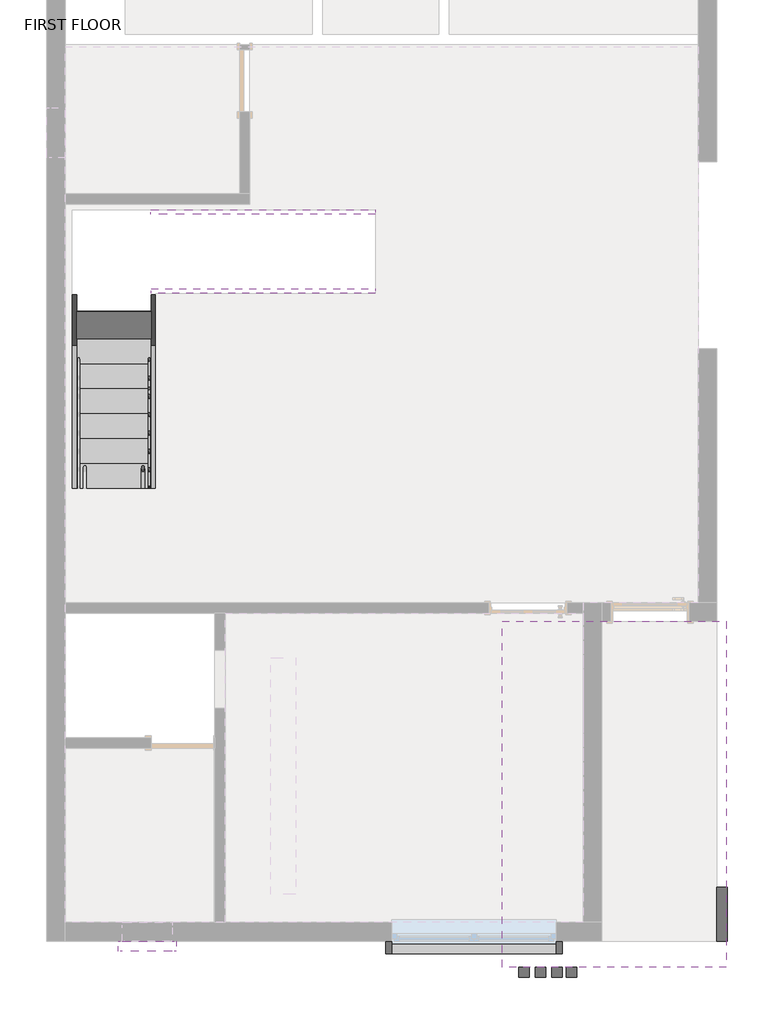
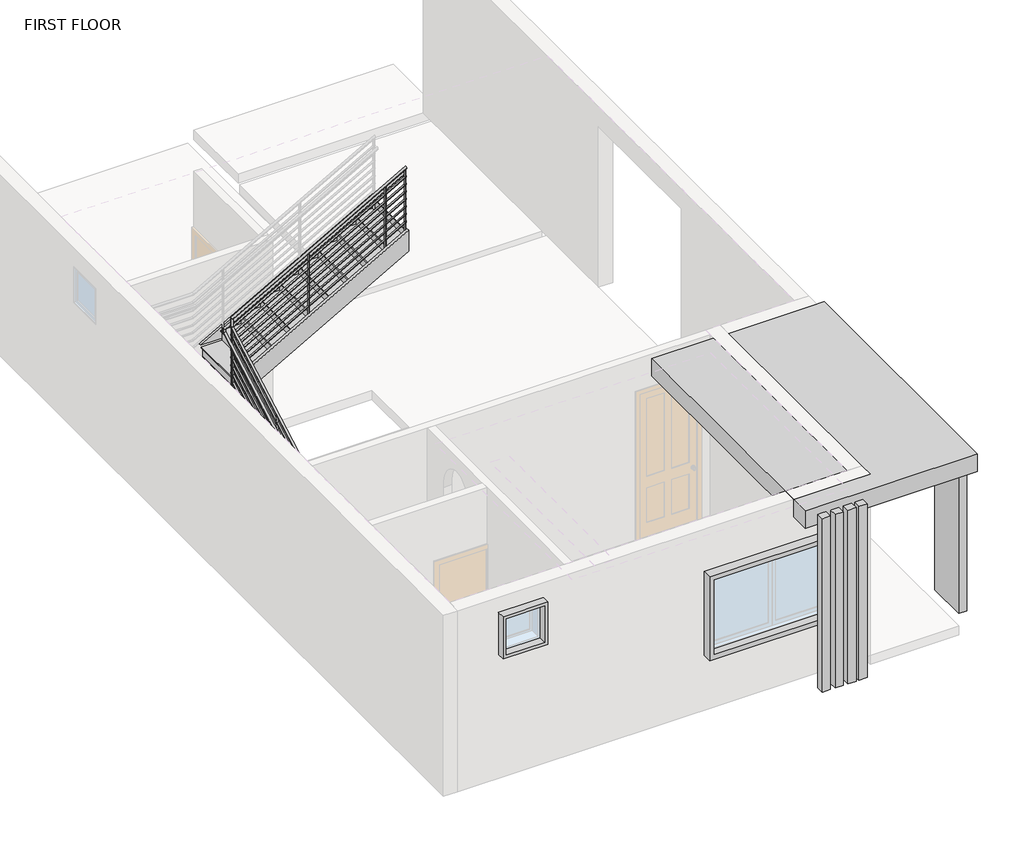
# One storey, part 3 of 3: 5 proxies, 4 members, 1 railing, 1 stair flight.
"""IFC4 building model written with IfcOpenShell, lengths in millimetres."""

from ifc_helpers import new_model, si_unit, frame, origin, place, context, project, spatial, polyline, circle_curve, ellipse_curve, outline, extrude, transform, mapped, element, save
from ifc_brep_helpers import plane_surface, cylinder_surface, advanced_brep
from components import generic_models_1_generic_models_1_e6ddf01a, generic_models_3_generic_models_3_ef4d42f5, generic_models_5_generic_models_5_8773877a, generic_models_7_generic_models_7_fd49988f, generic_models_9_generic_models_9_50e4b17c, stair_flight_ebba5fc4

model = new_model("IFC4")

# Units and contexts
model_context = context("Model", 3, world=origin())
ifc_project = project(units=[si_unit("LENGTHUNIT", "METRE", prefix="MILLI")], contexts=[model_context])

# Site, building, storey
site = spatial("IfcSite", under=ifc_project)
building = spatial("IfcBuilding", under=site)
storey = spatial("IfcBuildingStorey", under=building, Name="FIRST FLOOR", Elevation=3352.8)

# Proxies
placement = place(None, origin())
generic_models_1_generic_models_1_shape = generic_models_1_generic_models_1_e6ddf01a(model_context)
element("IfcBuildingElementProxy", 1, Name="Generic Models 1 : Generic Models 1", ObjectType="Generic Models 1 : Generic Models 1", at=placement, inside=storey, context=model_context, shape_type="MappedRepresentation", body=[
    mapped(generic_models_1_generic_models_1_shape, transform((0.0, 0.0, 0.0), x_axis=(1.0, 0.0, 0.0), y_axis=(0.0, 1.0, 0.0), z_axis=(0.0, 0.0, 1.0))),
])
generic_models_3_generic_models_3_shape = generic_models_3_generic_models_3_ef4d42f5(model_context)
element("IfcBuildingElementProxy", 2, Name="Generic Models 3 : Generic Models 3", ObjectType="Generic Models 3 : Generic Models 3", at=placement, inside=storey, context=model_context, shape_type="MappedRepresentation", body=[
    mapped(generic_models_3_generic_models_3_shape, transform((0.0, 0.0, 0.0), x_axis=(1.0, 0.0, 0.0), y_axis=(0.0, 1.0, 0.0), z_axis=(0.0, 0.0, 1.0))),
])
generic_models_5_generic_models_5_shape = generic_models_5_generic_models_5_8773877a(model_context)
element("IfcBuildingElementProxy", 3, Name="Generic Models 5 : Generic Models 5", ObjectType="Generic Models 5 : Generic Models 5", at=placement, inside=storey, context=model_context, shape_type="MappedRepresentation", body=[
    mapped(generic_models_5_generic_models_5_shape, transform((0.0, 0.0, 0.0), x_axis=(1.0, 0.0, 0.0), y_axis=(0.0, 1.0, 0.0), z_axis=(0.0, 0.0, 1.0))),
])
generic_models_7_generic_models_7_shape = generic_models_7_generic_models_7_fd49988f(model_context)
element("IfcBuildingElementProxy", 4, Name="Generic Models 7 : Generic Models 7", ObjectType="Generic Models 7 : Generic Models 7", at=placement, inside=storey, context=model_context, shape_type="MappedRepresentation", body=[
    mapped(generic_models_7_generic_models_7_shape, transform((0.0, 0.0, 0.0), x_axis=(1.0, 0.0, 0.0), y_axis=(0.0, 1.0, 0.0), z_axis=(0.0, 0.0, 1.0))),
])
generic_models_9_generic_models_9_shape = generic_models_9_generic_models_9_50e4b17c(model_context)
element("IfcBuildingElementProxy", 5, Name="Generic Models 9 : Generic Models 9", ObjectType="Generic Models 9 : Generic Models 9", at=placement, inside=storey, context=model_context, shape_type="MappedRepresentation", body=[
    mapped(generic_models_9_generic_models_9_shape, transform((0.0, 0.0, 0.0), x_axis=(1.0, 0.0, 0.0), y_axis=(0.0, 1.0, 0.0), z_axis=(0.0, 0.0, 1.0))),
])

# Members
element("IfcMember", 6, ObjectType="Stringer - 2\" Width", at=placement, inside=storey, context=model_context, shape_type="SweptSolid", body=[
    extrude(outline(polyline([(1771.427543, 3352.8), (1771.427543, 3561.3575825), (3600.227543, 4597.6775825), (4218.4673554, 4597.6775825), (2021.6245627, 3352.8), (1771.427543, 3352.8)])), frame((-6992.4757327, 0.0, 0.0), z_axis=(1.0, 0.0, 0.0), x_axis=(0.0, 1.0, 0.0)), (0.0, 0.0, 1.0), 50.8),
])
element("IfcMember", 7, ObjectType="Stringer - 2\" Width", at=placement, inside=storey, context=model_context, shape_type="SweptSolid", body=[
    extrude(outline(polyline([(5110.9416888, -5417.6757327), (6319.9816888, -3284.0757327), (6670.3175825, -3284.0757327), (5110.9416888, -6035.915545), (5110.9416888, -5417.6757327)])), frame((0.0, 5124.227543, 0.0), z_axis=(0.0, 1.0, 0.0), x_axis=(0.0, 0.0, 1.0)), (0.0, 0.0, 1.0), 50.8),
])
element("IfcMember", 8, ObjectType="Stringer - 2\" Width", at=placement, inside=storey, context=model_context, shape_type="SweptSolid", body=[
    extrude(outline(polyline([(1771.427543, 3352.8), (1771.427543, 3561.3575825), (4159.027543, 4914.3309158), (4159.027543, 4563.9950222), (2021.6245627, 3352.8), (1771.427543, 3352.8)])), frame((-6027.2757327, 0.0, 0.0), z_axis=(1.0, 0.0, 0.0), x_axis=(0.0, 1.0, 0.0)), (0.0, 0.0, 1.0), 50.8),
])
element("IfcMember", 9, ObjectType="Stringer - 2\" Width", at=placement, inside=storey, context=model_context, shape_type="SweptSolid", body=[
    extrude(outline(polyline([(5115.8375825, -6027.2757327), (4765.5016888, -6027.2757327), (6319.9816888, -3284.0757327), (6670.3175825, -3284.0757327), (5115.8375825, -6027.2757327)])), frame((0.0, 4159.027543, 0.0), z_axis=(0.0, 1.0, 0.0), x_axis=(0.0, 0.0, 1.0)), (0.0, 0.0, 1.0), 50.8),
])

# Railing
element("IfcRailing", 10, ObjectType="Guardrail - Pipe", at=placement, inside=storey, context=model_context, shape_type="AdvancedBrep", body=[
    advanced_brep(
    [(-6109.8257327, 1771.427543, 4418.0240066), (-6147.9257327, 1771.427543, 4418.0240066), (-6109.8257327, 4311.427543, 5857.35734), (-6147.9257327, 4311.427543, 5857.35734)],
    [
        (0, 1, ellipse_curve(frame((-6128.8757327, 1771.427543, 4418.0240066), z_axis=(0.0, -1.0, 0.0), x_axis=(0.0, 0.0, -0.9999999999999999)), 21.8959934, 19.05)),
        (1, 0, ellipse_curve(frame((-6128.8757327, 1771.427543, 4418.0240066), z_axis=(0.0, -1.0, 0.0), x_axis=(0.0, 0.0, -0.9999999999999999)), 21.8959934, 19.05)),
        (2, 3, ellipse_curve(frame((-6128.8757327, 4311.427543, 5857.35734), z_axis=(0.0, 0.5034815925230599, 0.864005952520261), x_axis=(0.0, -0.864005952520261, 0.5034815925230601)), 22.0484592, 19.05)),
        (3, 2, ellipse_curve(frame((-6128.8757327, 4311.427543, 5857.35734), z_axis=(0.0, 0.5034815925230599, 0.864005952520261), x_axis=(0.0, -0.864005952520261, 0.5034815925230601)), 22.0484592, 19.05)),
        (0, 2),
        (3, 1),
    ],
    [
        plane_surface(frame((-6128.8757327, 1771.427543, 4439.92), z_axis=(0.0, -1.0, 0.0), x_axis=(0.0, 0.0, 1.0))),
        plane_surface(frame((-6128.8757327, 4292.377543, 5868.4583333), z_axis=(0.0, 0.5034815925230599, 0.864005952520261), x_axis=(1.0, 0.0, 0.0))),
        cylinder_surface(frame((-6128.8757327, 1780.8194325, 4423.3460774), z_axis=(0.0, -0.8700221858486086, -0.49301257198088694), x_axis=(-1.0, 0.0, 0.0)), 19.05),
    ],
    [
        (0, [[1, 2]]),
        (1, [[3, 4]]),
        (2, [[-1, 5, -4, 6]]),
        (2, [[-2, -6, -3, -5]]),
    ],
),
    advanced_brep(
    [(-6109.8257327, 4313.9036203, 5855.9144571), (-6147.9257327, 4313.9036203, 5855.9144571), (-6109.8257327, 4313.9036203, 5903.82968), (-6147.9257327, 4313.9036203, 5926.0316667)],
    [
        (0, 1, ellipse_curve(frame((-6128.8757327, 4313.9036203, 5855.9144571), z_axis=(0.0, -0.5034815925230599, -0.864005952520261), x_axis=(0.0, 0.8640059525202612, -0.5034815925230599)), 22.0484592, 19.05)),
        (1, 0, ellipse_curve(frame((-6128.8757327, 4313.9036203, 5855.9144571), z_axis=(0.0, -0.5034815925230599, -0.864005952520261), x_axis=(0.0, 0.8640059525202612, -0.5034815925230599)), 22.0484592, 19.05)),
        (2, 3, ellipse_curve(frame((-6128.8757327, 4313.9036203, 5914.9306733), z_axis=(0.5034815925230599, 0.0, 0.864005952520261), x_axis=(0.8640059525202612, 0.0, -0.5034815925230599)), 22.0484592, 19.05)),
        (3, 2, ellipse_curve(frame((-6128.8757327, 4313.9036203, 5914.9306733), z_axis=(0.5034815925230599, 0.0, 0.864005952520261), x_axis=(0.8640059525202612, 0.0, -0.5034815925230599)), 22.0484592, 19.05)),
        (0, 2),
        (3, 1),
    ],
    [
        plane_surface(frame((-6128.8757327, 4311.427543, 5857.35734), z_axis=(0.0, -0.5034815925230599, -0.864005952520261), x_axis=(1.0, 0.0, 0.0))),
        plane_surface(frame((-6128.8757327, 4311.427543, 5914.9306733), z_axis=(0.5034815925230599, 0.0, 0.864005952520261), x_axis=(0.864005952520261, 0.0, -0.5034815925230599))),
        cylinder_surface(frame((-6128.8757327, 4313.9036203, 5857.35734), z_axis=(0.0, 0.0, -1.0), x_axis=(-1.0, 0.0, 0.0)), 19.05),
    ],
    [
        (0, [[1, 2]]),
        (1, [[3, 4]]),
        (2, [[-1, 5, -4, 6]]),
        (2, [[-2, -6, -3, -5]]),
    ],
),
    advanced_brep(
    [(-6128.8757327, 4292.377543, 5914.9306733), (-6128.8757327, 4330.477543, 5914.9306733), (-3284.0757327, 4292.377543, 7526.9840066), (-3284.0757327, 4330.477543, 7526.9840066)],
    [
        (0, 1, ellipse_curve(frame((-6128.8757327, 4311.427543, 5914.9306733), z_axis=(-0.5034815925230599, 0.0, -0.864005952520261), x_axis=(-0.864005952520261, 0.0, 0.5034815925230601)), 22.0484592, 19.05)),
        (1, 0, ellipse_curve(frame((-6128.8757327, 4311.427543, 5914.9306733), z_axis=(-0.5034815925230599, 0.0, -0.864005952520261), x_axis=(-0.864005952520261, 0.0, 0.5034815925230601)), 22.0484592, 19.05)),
        (2, 3, ellipse_curve(frame((-3284.0757327, 4311.427543, 7526.9840066), z_axis=(1.0, 0.0, 0.0), x_axis=(0.0, 0.0, -0.9999999999999999)), 21.8959934, 19.05)),
        (3, 2, ellipse_curve(frame((-3284.0757327, 4311.427543, 7526.9840066), z_axis=(1.0, 0.0, 0.0), x_axis=(0.0, 0.0, -0.9999999999999999)), 21.8959934, 19.05)),
        (0, 2),
        (3, 1),
    ],
    [
        plane_surface(frame((-6147.9257327, 4311.427543, 5926.0316667), z_axis=(-0.5034815925230599, 0.0, -0.864005952520261), x_axis=(0.864005952520261, 0.0, -0.5034815925230599))),
        plane_surface(frame((-3284.0757327, 4311.427543, 7548.88), z_axis=(1.0, 0.0, 0.0), x_axis=(0.0, 1.0, 0.0))),
        cylinder_surface(frame((-6138.5338432, 4311.427543, 5909.457744), z_axis=(-0.8700221858486086, 0.0, -0.49301257198088694), x_axis=(0.0, 1.0, 0.0)), 19.05),
    ],
    [
        (0, [[1, 2]]),
        (1, [[3, 4]]),
        (2, [[-1, 5, -4, 6]]),
        (2, [[-2, -6, -3, -5]]),
    ],
),
    advanced_brep(
    [(-6033.6257327, 1771.427543, 4570.4240066), (-6071.7257327, 1771.427543, 4570.4240066), (-6033.6257327, 4235.227543, 5966.57734), (-6071.7257327, 4235.227543, 5966.57734)],
    [
        (0, 1, ellipse_curve(frame((-6052.6757327, 1771.427543, 4570.4240066), z_axis=(0.0, -1.0, 0.0), x_axis=(0.0, 0.0, -0.9999999999999999)), 21.8959934, 19.05)),
        (1, 0, ellipse_curve(frame((-6052.6757327, 1771.427543, 4570.4240066), z_axis=(0.0, -1.0, 0.0), x_axis=(0.0, 0.0, -0.9999999999999999)), 21.8959934, 19.05)),
        (2, 3, ellipse_curve(frame((-6052.6757327, 4235.227543, 5966.57734), z_axis=(0.0, 0.5034815925230599, 0.864005952520261), x_axis=(0.0, -0.864005952520261, 0.5034815925230601)), 22.0484592, 19.05)),
        (3, 2, ellipse_curve(frame((-6052.6757327, 4235.227543, 5966.57734), z_axis=(0.0, 0.5034815925230599, 0.864005952520261), x_axis=(0.0, -0.864005952520261, 0.5034815925230601)), 22.0484592, 19.05)),
        (0, 2),
        (3, 1),
    ],
    [
        plane_surface(frame((-6052.6757327, 1771.427543, 4592.32), z_axis=(0.0, -1.0, 0.0), x_axis=(0.0, 0.0, 1.0))),
        plane_surface(frame((-6052.6757327, 4216.177543, 5977.6783333), z_axis=(0.0, 0.5034815925230599, 0.864005952520261), x_axis=(1.0, 0.0, 0.0))),
        cylinder_surface(frame((-6052.6757327, 1780.8194325, 4575.7460774), z_axis=(0.0, -0.8700221858486086, -0.49301257198088694), x_axis=(-1.0, 0.0, 0.0)), 19.05),
    ],
    [
        (0, [[1, 2]]),
        (1, [[3, 4]]),
        (2, [[-1, 5, -4, 6]]),
        (2, [[-2, -6, -3, -5]]),
    ],
),
    advanced_brep(
    [(-6033.6257327, 4237.7036203, 5965.1344571), (-6071.7257327, 4237.7036203, 5965.1344571), (-6033.6257327, 4237.7036203, 6099.40968), (-6071.7257327, 4237.7036203, 6121.6116667)],
    [
        (0, 1, ellipse_curve(frame((-6052.6757327, 4237.7036203, 5965.1344571), z_axis=(0.0, -0.5034815925230599, -0.864005952520261), x_axis=(0.0, 0.8640059525202612, -0.5034815925230599)), 22.0484592, 19.05)),
        (1, 0, ellipse_curve(frame((-6052.6757327, 4237.7036203, 5965.1344571), z_axis=(0.0, -0.5034815925230599, -0.864005952520261), x_axis=(0.0, 0.8640059525202612, -0.5034815925230599)), 22.0484592, 19.05)),
        (2, 3, ellipse_curve(frame((-6052.6757327, 4237.7036203, 6110.5106733), z_axis=(0.5034815925230599, 0.0, 0.864005952520261), x_axis=(0.8640059525202612, 0.0, -0.5034815925230599)), 22.0484592, 19.05)),
        (3, 2, ellipse_curve(frame((-6052.6757327, 4237.7036203, 6110.5106733), z_axis=(0.5034815925230599, 0.0, 0.864005952520261), x_axis=(0.8640059525202612, 0.0, -0.5034815925230599)), 22.0484592, 19.05)),
        (0, 2),
        (3, 1),
    ],
    [
        plane_surface(frame((-6052.6757327, 4235.227543, 5966.57734), z_axis=(0.0, -0.5034815925230599, -0.864005952520261), x_axis=(1.0, 0.0, 0.0))),
        plane_surface(frame((-6052.6757327, 4235.227543, 6110.5106733), z_axis=(0.5034815925230599, 0.0, 0.864005952520261), x_axis=(0.864005952520261, 0.0, -0.5034815925230599))),
        cylinder_surface(frame((-6052.6757327, 4237.7036203, 5966.57734), z_axis=(0.0, 0.0, -1.0), x_axis=(-1.0, 0.0, 0.0)), 19.05),
    ],
    [
        (0, [[1, 2]]),
        (1, [[3, 4]]),
        (2, [[-1, 5, -4, 6]]),
        (2, [[-2, -6, -3, -5]]),
    ],
),
    advanced_brep(
    [(-6052.6757327, 4216.177543, 6110.5106733), (-6052.6757327, 4254.277543, 6110.5106733), (-3284.0757327, 4216.177543, 7679.3840066), (-3284.0757327, 4254.277543, 7679.3840066)],
    [
        (0, 1, ellipse_curve(frame((-6052.6757327, 4235.227543, 6110.5106733), z_axis=(-0.5034815925230599, 0.0, -0.864005952520261), x_axis=(-0.864005952520261, 0.0, 0.5034815925230601)), 22.0484592, 19.05)),
        (1, 0, ellipse_curve(frame((-6052.6757327, 4235.227543, 6110.5106733), z_axis=(-0.5034815925230599, 0.0, -0.864005952520261), x_axis=(-0.864005952520261, 0.0, 0.5034815925230601)), 22.0484592, 19.05)),
        (2, 3, ellipse_curve(frame((-3284.0757327, 4235.227543, 7679.3840066), z_axis=(1.0, 0.0, 0.0), x_axis=(0.0, 0.0, -0.9999999999999999)), 21.8959934, 19.05)),
        (3, 2, ellipse_curve(frame((-3284.0757327, 4235.227543, 7679.3840066), z_axis=(1.0, 0.0, 0.0), x_axis=(0.0, 0.0, -0.9999999999999999)), 21.8959934, 19.05)),
        (0, 2),
        (3, 1),
    ],
    [
        plane_surface(frame((-6071.7257327, 4235.227543, 6121.6116667), z_axis=(-0.5034815925230599, 0.0, -0.864005952520261), x_axis=(0.864005952520261, 0.0, -0.5034815925230599))),
        plane_surface(frame((-3284.0757327, 4235.227543, 7701.28), z_axis=(1.0, 0.0, 0.0), x_axis=(0.0, 1.0, 0.0))),
        cylinder_surface(frame((-6062.3338432, 4235.227543, 6105.037744), z_axis=(-0.8700221858486086, 0.0, -0.49301257198088694), x_axis=(0.0, 1.0, 0.0)), 19.05),
    ],
    [
        (0, [[1, 2]]),
        (1, [[3, 4]]),
        (2, [[-1, 5, -4, 6]]),
        (2, [[-2, -6, -3, -5]]),
    ],
),
    advanced_brep(
    [(-6065.3757327, 1771.427543, 4425.3226711), (-6039.9757327, 1771.427543, 4425.3226711), (-6065.3757327, 4222.527543, 5814.2793378), (-6039.9757327, 4222.527543, 5814.2793378)],
    [
        (0, 1, ellipse_curve(frame((-6052.6757327, 1771.427543, 4425.3226711), z_axis=(0.0, -1.0, 0.0), x_axis=(0.0, 0.0, -0.9999999999999999)), 14.5973289, 12.7)),
        (1, 0, ellipse_curve(frame((-6052.6757327, 1771.427543, 4425.3226711), z_axis=(0.0, -1.0, 0.0), x_axis=(0.0, 0.0, -0.9999999999999999)), 14.5973289, 12.7)),
        (2, 3, ellipse_curve(frame((-6052.6757327, 4222.527543, 5814.2793378), z_axis=(0.0, 1.0, 0.0), x_axis=(0.0, 0.0, -0.9999999999999999)), 14.5973289, 12.7)),
        (3, 2, ellipse_curve(frame((-6052.6757327, 4222.527543, 5814.2793378), z_axis=(0.0, 1.0, 0.0), x_axis=(0.0, 0.0, -0.9999999999999999)), 14.5973289, 12.7)),
        (0, 2),
        (3, 1),
    ],
    [
        plane_surface(frame((-6052.6757327, 1771.427543, 4439.92), z_axis=(0.0, -1.0, 0.0), x_axis=(0.0, 0.0, 1.0))),
        plane_surface(frame((-6052.6757327, 4222.527543, 5828.8766667), z_axis=(0.0, 1.0, 0.0), x_axis=(0.0, 0.0, 1.0))),
        cylinder_surface(frame((-6052.6757327, 1777.6888026, 4428.8707182), z_axis=(0.0, -0.8700221858486086, -0.49301257198088694), x_axis=(1.0, 0.0, 0.0)), 12.7),
    ],
    [
        (0, [[1, 2]]),
        (1, [[3, 4]]),
        (2, [[-1, 5, -4, 6]]),
        (2, [[-2, -6, -3, -5]]),
    ],
),
    advanced_brep(
    [(-6065.3757327, 4247.927543, 5958.2126711), (-6065.3757327, 4222.527543, 5958.2126711), (-3284.0757327, 4247.927543, 7534.2826711), (-3284.0757327, 4222.527543, 7534.2826711)],
    [
        (0, 1, ellipse_curve(frame((-6065.3757327, 4235.227543, 5958.2126711), z_axis=(-1.0, 0.0, 0.0), x_axis=(0.0, 0.0, -0.9999999999999999)), 14.5973289, 12.7)),
        (1, 0, ellipse_curve(frame((-6065.3757327, 4235.227543, 5958.2126711), z_axis=(-1.0, 0.0, 0.0), x_axis=(0.0, 0.0, -0.9999999999999999)), 14.5973289, 12.7)),
        (2, 3, ellipse_curve(frame((-3284.0757327, 4235.227543, 7534.2826711), z_axis=(1.0, 0.0, 0.0), x_axis=(0.0, 0.0, -0.9999999999999999)), 14.5973289, 12.7)),
        (3, 2, ellipse_curve(frame((-3284.0757327, 4235.227543, 7534.2826711), z_axis=(1.0, 0.0, 0.0), x_axis=(0.0, 0.0, -0.9999999999999999)), 14.5973289, 12.7)),
        (0, 2),
        (3, 1),
    ],
    [
        plane_surface(frame((-6065.3757327, 4235.227543, 5972.81), z_axis=(-1.0, 0.0, 0.0), x_axis=(0.0, 1.0, 0.0))),
        plane_surface(frame((-3284.0757327, 4235.227543, 7548.88), z_axis=(1.0, 0.0, 0.0), x_axis=(0.0, 1.0, 0.0))),
        cylinder_surface(frame((-6059.114473, 4235.227543, 5961.7607182), z_axis=(-0.8700221858486086, 0.0, -0.49301257198088694), x_axis=(0.0, -1.0, 0.0)), 12.7),
    ],
    [
        (0, [[1, 2]]),
        (1, [[3, 4]]),
        (2, [[-1, 5, -4, 6]]),
        (2, [[-2, -6, -3, -5]]),
    ],
),
    advanced_brep(
    [(-6065.3757327, 1771.427543, 4298.3226711), (-6039.9757327, 1771.427543, 4298.3226711), (-6065.3757327, 4222.527543, 5687.2793378), (-6039.9757327, 4222.527543, 5687.2793378)],
    [
        (0, 1, ellipse_curve(frame((-6052.6757327, 1771.427543, 4298.3226711), z_axis=(0.0, -1.0, 0.0), x_axis=(0.0, 0.0, -0.9999999999999999)), 14.5973289, 12.7)),
        (1, 0, ellipse_curve(frame((-6052.6757327, 1771.427543, 4298.3226711), z_axis=(0.0, -1.0, 0.0), x_axis=(0.0, 0.0, -0.9999999999999999)), 14.5973289, 12.7)),
        (2, 3, ellipse_curve(frame((-6052.6757327, 4222.527543, 5687.2793378), z_axis=(0.0, 1.0, 0.0), x_axis=(0.0, 0.0, -0.9999999999999999)), 14.5973289, 12.7)),
        (3, 2, ellipse_curve(frame((-6052.6757327, 4222.527543, 5687.2793378), z_axis=(0.0, 1.0, 0.0), x_axis=(0.0, 0.0, -0.9999999999999999)), 14.5973289, 12.7)),
        (0, 2),
        (3, 1),
    ],
    [
        plane_surface(frame((-6052.6757327, 1771.427543, 4312.92), z_axis=(0.0, -1.0, 0.0), x_axis=(0.0, 0.0, 1.0))),
        plane_surface(frame((-6052.6757327, 4222.527543, 5701.8766667), z_axis=(0.0, 1.0, 0.0), x_axis=(0.0, 0.0, 1.0))),
        cylinder_surface(frame((-6052.6757327, 1777.6888026, 4301.8707182), z_axis=(0.0, -0.8700221858486086, -0.49301257198088694), x_axis=(1.0, 0.0, 0.0)), 12.7),
    ],
    [
        (0, [[1, 2]]),
        (1, [[3, 4]]),
        (2, [[-1, 5, -4, 6]]),
        (2, [[-2, -6, -3, -5]]),
    ],
),
    advanced_brep(
    [(-6065.3757327, 4247.927543, 5831.2126711), (-6065.3757327, 4222.527543, 5831.2126711), (-3284.0757327, 4247.927543, 7407.2826711), (-3284.0757327, 4222.527543, 7407.2826711)],
    [
        (0, 1, ellipse_curve(frame((-6065.3757327, 4235.227543, 5831.2126711), z_axis=(-1.0, 0.0, 0.0), x_axis=(0.0, 0.0, -0.9999999999999999)), 14.5973289, 12.7)),
        (1, 0, ellipse_curve(frame((-6065.3757327, 4235.227543, 5831.2126711), z_axis=(-1.0, 0.0, 0.0), x_axis=(0.0, 0.0, -0.9999999999999999)), 14.5973289, 12.7)),
        (2, 3, ellipse_curve(frame((-3284.0757327, 4235.227543, 7407.2826711), z_axis=(1.0, 0.0, 0.0), x_axis=(0.0, 0.0, -0.9999999999999999)), 14.5973289, 12.7)),
        (3, 2, ellipse_curve(frame((-3284.0757327, 4235.227543, 7407.2826711), z_axis=(1.0, 0.0, 0.0), x_axis=(0.0, 0.0, -0.9999999999999999)), 14.5973289, 12.7)),
        (0, 2),
        (3, 1),
    ],
    [
        plane_surface(frame((-6065.3757327, 4235.227543, 5845.81), z_axis=(-1.0, 0.0, 0.0), x_axis=(0.0, 1.0, 0.0))),
        plane_surface(frame((-3284.0757327, 4235.227543, 7421.88), z_axis=(1.0, 0.0, 0.0), x_axis=(0.0, 1.0, 0.0))),
        cylinder_surface(frame((-6059.114473, 4235.227543, 5834.7607182), z_axis=(-0.8700221858486086, 0.0, -0.49301257198088694), x_axis=(0.0, -1.0, 0.0)), 12.7),
    ],
    [
        (0, [[1, 2]]),
        (1, [[3, 4]]),
        (2, [[-1, 5, -4, 6]]),
        (2, [[-2, -6, -3, -5]]),
    ],
),
    advanced_brep(
    [(-6065.3757327, 1771.427543, 4171.3226711), (-6039.9757327, 1771.427543, 4171.3226711), (-6065.3757327, 4222.527543, 5560.2793378), (-6039.9757327, 4222.527543, 5560.2793378)],
    [
        (0, 1, ellipse_curve(frame((-6052.6757327, 1771.427543, 4171.3226711), z_axis=(0.0, -1.0, 0.0), x_axis=(0.0, 0.0, -0.9999999999999999)), 14.5973289, 12.7)),
        (1, 0, ellipse_curve(frame((-6052.6757327, 1771.427543, 4171.3226711), z_axis=(0.0, -1.0, 0.0), x_axis=(0.0, 0.0, -0.9999999999999999)), 14.5973289, 12.7)),
        (2, 3, ellipse_curve(frame((-6052.6757327, 4222.527543, 5560.2793378), z_axis=(0.0, 1.0, 0.0), x_axis=(0.0, 0.0, -0.9999999999999999)), 14.5973289, 12.7)),
        (3, 2, ellipse_curve(frame((-6052.6757327, 4222.527543, 5560.2793378), z_axis=(0.0, 1.0, 0.0), x_axis=(0.0, 0.0, -0.9999999999999999)), 14.5973289, 12.7)),
        (0, 2),
        (3, 1),
    ],
    [
        plane_surface(frame((-6052.6757327, 1771.427543, 4185.92), z_axis=(0.0, -1.0, 0.0), x_axis=(0.0, 0.0, 1.0))),
        plane_surface(frame((-6052.6757327, 4222.527543, 5574.8766667), z_axis=(0.0, 1.0, 0.0), x_axis=(0.0, 0.0, 1.0))),
        cylinder_surface(frame((-6052.6757327, 1777.6888026, 4174.8707182), z_axis=(0.0, -0.8700221858486086, -0.49301257198088694), x_axis=(1.0, 0.0, 0.0)), 12.7),
    ],
    [
        (0, [[1, 2]]),
        (1, [[3, 4]]),
        (2, [[-1, 5, -4, 6]]),
        (2, [[-2, -6, -3, -5]]),
    ],
),
    advanced_brep(
    [(-6065.3757327, 4247.927543, 5704.2126711), (-6065.3757327, 4222.527543, 5704.2126711), (-3284.0757327, 4247.927543, 7280.2826711), (-3284.0757327, 4222.527543, 7280.2826711)],
    [
        (0, 1, ellipse_curve(frame((-6065.3757327, 4235.227543, 5704.2126711), z_axis=(-1.0, 0.0, 0.0), x_axis=(0.0, 0.0, -0.9999999999999999)), 14.5973289, 12.7)),
        (1, 0, ellipse_curve(frame((-6065.3757327, 4235.227543, 5704.2126711), z_axis=(-1.0, 0.0, 0.0), x_axis=(0.0, 0.0, -0.9999999999999999)), 14.5973289, 12.7)),
        (2, 3, ellipse_curve(frame((-3284.0757327, 4235.227543, 7280.2826711), z_axis=(1.0, 0.0, 0.0), x_axis=(0.0, 0.0, -0.9999999999999999)), 14.5973289, 12.7)),
        (3, 2, ellipse_curve(frame((-3284.0757327, 4235.227543, 7280.2826711), z_axis=(1.0, 0.0, 0.0), x_axis=(0.0, 0.0, -0.9999999999999999)), 14.5973289, 12.7)),
        (0, 2),
        (3, 1),
    ],
    [
        plane_surface(frame((-6065.3757327, 4235.227543, 5718.81), z_axis=(-1.0, 0.0, 0.0), x_axis=(0.0, 1.0, 0.0))),
        plane_surface(frame((-3284.0757327, 4235.227543, 7294.88), z_axis=(1.0, 0.0, 0.0), x_axis=(0.0, 1.0, 0.0))),
        cylinder_surface(frame((-6059.114473, 4235.227543, 5707.7607182), z_axis=(-0.8700221858486086, 0.0, -0.49301257198088694), x_axis=(0.0, -1.0, 0.0)), 12.7),
    ],
    [
        (0, [[1, 2]]),
        (1, [[3, 4]]),
        (2, [[-1, 5, -4, 6]]),
        (2, [[-2, -6, -3, -5]]),
    ],
),
    advanced_brep(
    [(-6065.3757327, 1771.427543, 4044.3226711), (-6039.9757327, 1771.427543, 4044.3226711), (-6065.3757327, 4222.527543, 5433.2793378), (-6039.9757327, 4222.527543, 5433.2793378)],
    [
        (0, 1, ellipse_curve(frame((-6052.6757327, 1771.427543, 4044.3226711), z_axis=(0.0, -1.0, 0.0), x_axis=(0.0, 0.0, -0.9999999999999999)), 14.5973289, 12.7)),
        (1, 0, ellipse_curve(frame((-6052.6757327, 1771.427543, 4044.3226711), z_axis=(0.0, -1.0, 0.0), x_axis=(0.0, 0.0, -0.9999999999999999)), 14.5973289, 12.7)),
        (2, 3, ellipse_curve(frame((-6052.6757327, 4222.527543, 5433.2793378), z_axis=(0.0, 1.0, 0.0), x_axis=(0.0, 0.0, -0.9999999999999999)), 14.5973289, 12.7)),
        (3, 2, ellipse_curve(frame((-6052.6757327, 4222.527543, 5433.2793378), z_axis=(0.0, 1.0, 0.0), x_axis=(0.0, 0.0, -0.9999999999999999)), 14.5973289, 12.7)),
        (0, 2),
        (3, 1),
    ],
    [
        plane_surface(frame((-6052.6757327, 1771.427543, 4058.92), z_axis=(0.0, -1.0, 0.0), x_axis=(0.0, 0.0, 1.0))),
        plane_surface(frame((-6052.6757327, 4222.527543, 5447.8766667), z_axis=(0.0, 1.0, 0.0), x_axis=(0.0, 0.0, 1.0))),
        cylinder_surface(frame((-6052.6757327, 1777.6888026, 4047.8707182), z_axis=(0.0, -0.8700221858486086, -0.49301257198088694), x_axis=(1.0, 0.0, 0.0)), 12.7),
    ],
    [
        (0, [[1, 2]]),
        (1, [[3, 4]]),
        (2, [[-1, 5, -4, 6]]),
        (2, [[-2, -6, -3, -5]]),
    ],
),
    advanced_brep(
    [(-6065.3757327, 4247.927543, 5577.2126711), (-6065.3757327, 4222.527543, 5577.2126711), (-3284.0757327, 4247.927543, 7153.2826711), (-3284.0757327, 4222.527543, 7153.2826711)],
    [
        (0, 1, ellipse_curve(frame((-6065.3757327, 4235.227543, 5577.2126711), z_axis=(-1.0, 0.0, 0.0), x_axis=(0.0, 0.0, -0.9999999999999999)), 14.5973289, 12.7)),
        (1, 0, ellipse_curve(frame((-6065.3757327, 4235.227543, 5577.2126711), z_axis=(-1.0, 0.0, 0.0), x_axis=(0.0, 0.0, -0.9999999999999999)), 14.5973289, 12.7)),
        (2, 3, ellipse_curve(frame((-3284.0757327, 4235.227543, 7153.2826711), z_axis=(1.0, 0.0, 0.0), x_axis=(0.0, 0.0, -0.9999999999999999)), 14.5973289, 12.7)),
        (3, 2, ellipse_curve(frame((-3284.0757327, 4235.227543, 7153.2826711), z_axis=(1.0, 0.0, 0.0), x_axis=(0.0, 0.0, -0.9999999999999999)), 14.5973289, 12.7)),
        (0, 2),
        (3, 1),
    ],
    [
        plane_surface(frame((-6065.3757327, 4235.227543, 5591.81), z_axis=(-1.0, 0.0, 0.0), x_axis=(0.0, 1.0, 0.0))),
        plane_surface(frame((-3284.0757327, 4235.227543, 7167.88), z_axis=(1.0, 0.0, 0.0), x_axis=(0.0, 1.0, 0.0))),
        cylinder_surface(frame((-6059.114473, 4235.227543, 5580.7607182), z_axis=(-0.8700221858486086, 0.0, -0.49301257198088694), x_axis=(0.0, -1.0, 0.0)), 12.7),
    ],
    [
        (0, [[1, 2]]),
        (1, [[3, 4]]),
        (2, [[-1, 5, -4, 6]]),
        (2, [[-2, -6, -3, -5]]),
    ],
),
    advanced_brep(
    [(-6065.3757327, 1771.427543, 3917.3226711), (-6039.9757327, 1771.427543, 3917.3226711), (-6065.3757327, 4222.527543, 5306.2793378), (-6039.9757327, 4222.527543, 5306.2793378)],
    [
        (0, 1, ellipse_curve(frame((-6052.6757327, 1771.427543, 3917.3226711), z_axis=(0.0, -1.0, 0.0), x_axis=(0.0, 0.0, -0.9999999999999999)), 14.5973289, 12.7)),
        (1, 0, ellipse_curve(frame((-6052.6757327, 1771.427543, 3917.3226711), z_axis=(0.0, -1.0, 0.0), x_axis=(0.0, 0.0, -0.9999999999999999)), 14.5973289, 12.7)),
        (2, 3, ellipse_curve(frame((-6052.6757327, 4222.527543, 5306.2793378), z_axis=(0.0, 1.0, 0.0), x_axis=(0.0, 0.0, -0.9999999999999999)), 14.5973289, 12.7)),
        (3, 2, ellipse_curve(frame((-6052.6757327, 4222.527543, 5306.2793378), z_axis=(0.0, 1.0, 0.0), x_axis=(0.0, 0.0, -0.9999999999999999)), 14.5973289, 12.7)),
        (0, 2),
        (3, 1),
    ],
    [
        plane_surface(frame((-6052.6757327, 1771.427543, 3931.92), z_axis=(0.0, -1.0, 0.0), x_axis=(0.0, 0.0, 1.0))),
        plane_surface(frame((-6052.6757327, 4222.527543, 5320.8766667), z_axis=(0.0, 1.0, 0.0), x_axis=(0.0, 0.0, 1.0))),
        cylinder_surface(frame((-6052.6757327, 1777.6888026, 3920.8707182), z_axis=(0.0, -0.8700221858486086, -0.49301257198088694), x_axis=(1.0, 0.0, 0.0)), 12.7),
    ],
    [
        (0, [[1, 2]]),
        (1, [[3, 4]]),
        (2, [[-1, 5, -4, 6]]),
        (2, [[-2, -6, -3, -5]]),
    ],
),
    advanced_brep(
    [(-6065.3757327, 4247.927543, 5450.2126711), (-6065.3757327, 4222.527543, 5450.2126711), (-3284.0757327, 4247.927543, 7026.2826711), (-3284.0757327, 4222.527543, 7026.2826711)],
    [
        (0, 1, ellipse_curve(frame((-6065.3757327, 4235.227543, 5450.2126711), z_axis=(-1.0, 0.0, 0.0), x_axis=(0.0, 0.0, -0.9999999999999999)), 14.5973289, 12.7)),
        (1, 0, ellipse_curve(frame((-6065.3757327, 4235.227543, 5450.2126711), z_axis=(-1.0, 0.0, 0.0), x_axis=(0.0, 0.0, -0.9999999999999999)), 14.5973289, 12.7)),
        (2, 3, ellipse_curve(frame((-3284.0757327, 4235.227543, 7026.2826711), z_axis=(1.0, 0.0, 0.0), x_axis=(0.0, 0.0, -0.9999999999999999)), 14.5973289, 12.7)),
        (3, 2, ellipse_curve(frame((-3284.0757327, 4235.227543, 7026.2826711), z_axis=(1.0, 0.0, 0.0), x_axis=(0.0, 0.0, -0.9999999999999999)), 14.5973289, 12.7)),
        (0, 2),
        (3, 1),
    ],
    [
        plane_surface(frame((-6065.3757327, 4235.227543, 5464.81), z_axis=(-1.0, 0.0, 0.0), x_axis=(0.0, 1.0, 0.0))),
        plane_surface(frame((-3284.0757327, 4235.227543, 7040.88), z_axis=(1.0, 0.0, 0.0), x_axis=(0.0, 1.0, 0.0))),
        cylinder_surface(frame((-6059.114473, 4235.227543, 5453.7607182), z_axis=(-0.8700221858486086, 0.0, -0.49301257198088694), x_axis=(0.0, -1.0, 0.0)), 12.7),
    ],
    [
        (0, [[1, 2]]),
        (1, [[3, 4]]),
        (2, [[-1, 5, -4, 6]]),
        (2, [[-2, -6, -3, -5]]),
    ],
),
    advanced_brep(
    [(-6065.3757327, 1771.427543, 3790.3226711), (-6039.9757327, 1771.427543, 3790.3226711), (-6065.3757327, 4222.527543, 5179.2793378), (-6039.9757327, 4222.527543, 5179.2793378)],
    [
        (0, 1, ellipse_curve(frame((-6052.6757327, 1771.427543, 3790.3226711), z_axis=(0.0, -1.0, 0.0), x_axis=(0.0, 0.0, -0.9999999999999999)), 14.5973289, 12.7)),
        (1, 0, ellipse_curve(frame((-6052.6757327, 1771.427543, 3790.3226711), z_axis=(0.0, -1.0, 0.0), x_axis=(0.0, 0.0, -0.9999999999999999)), 14.5973289, 12.7)),
        (2, 3, ellipse_curve(frame((-6052.6757327, 4222.527543, 5179.2793378), z_axis=(0.0, 1.0, 0.0), x_axis=(0.0, 0.0, -0.9999999999999999)), 14.5973289, 12.7)),
        (3, 2, ellipse_curve(frame((-6052.6757327, 4222.527543, 5179.2793378), z_axis=(0.0, 1.0, 0.0), x_axis=(0.0, 0.0, -0.9999999999999999)), 14.5973289, 12.7)),
        (0, 2),
        (3, 1),
    ],
    [
        plane_surface(frame((-6052.6757327, 1771.427543, 3804.92), z_axis=(0.0, -1.0, 0.0), x_axis=(0.0, 0.0, 1.0))),
        plane_surface(frame((-6052.6757327, 4222.527543, 5193.8766667), z_axis=(0.0, 1.0, 0.0), x_axis=(0.0, 0.0, 1.0))),
        cylinder_surface(frame((-6052.6757327, 1777.6888026, 3793.8707182), z_axis=(0.0, -0.8700221858486086, -0.49301257198088694), x_axis=(1.0, 0.0, 0.0)), 12.7),
    ],
    [
        (0, [[1, 2]]),
        (1, [[3, 4]]),
        (2, [[-1, 5, -4, 6]]),
        (2, [[-2, -6, -3, -5]]),
    ],
),
    advanced_brep(
    [(-6065.3757327, 4247.927543, 5323.2126711), (-6065.3757327, 4222.527543, 5323.2126711), (-3284.0757327, 4247.927543, 6899.2826711), (-3284.0757327, 4222.527543, 6899.2826711)],
    [
        (0, 1, ellipse_curve(frame((-6065.3757327, 4235.227543, 5323.2126711), z_axis=(-1.0, 0.0, 0.0), x_axis=(0.0, 0.0, -0.9999999999999999)), 14.5973289, 12.7)),
        (1, 0, ellipse_curve(frame((-6065.3757327, 4235.227543, 5323.2126711), z_axis=(-1.0, 0.0, 0.0), x_axis=(0.0, 0.0, -0.9999999999999999)), 14.5973289, 12.7)),
        (2, 3, ellipse_curve(frame((-3284.0757327, 4235.227543, 6899.2826711), z_axis=(1.0, 0.0, 0.0), x_axis=(0.0, 0.0, -0.9999999999999999)), 14.5973289, 12.7)),
        (3, 2, ellipse_curve(frame((-3284.0757327, 4235.227543, 6899.2826711), z_axis=(1.0, 0.0, 0.0), x_axis=(0.0, 0.0, -0.9999999999999999)), 14.5973289, 12.7)),
        (0, 2),
        (3, 1),
    ],
    [
        plane_surface(frame((-6065.3757327, 4235.227543, 5337.81), z_axis=(-1.0, 0.0, 0.0), x_axis=(0.0, 1.0, 0.0))),
        plane_surface(frame((-3284.0757327, 4235.227543, 6913.88), z_axis=(1.0, 0.0, 0.0), x_axis=(0.0, 1.0, 0.0))),
        cylinder_surface(frame((-6059.114473, 4235.227543, 5326.7607182), z_axis=(-0.8700221858486086, 0.0, -0.49301257198088694), x_axis=(0.0, -1.0, 0.0)), 12.7),
    ],
    [
        (0, [[1, 2]]),
        (1, [[3, 4]]),
        (2, [[-1, 5, -4, 6]]),
        (2, [[-2, -6, -3, -5]]),
    ],
),
    advanced_brep(
    [(-6065.3757327, 1771.427543, 3663.3226711), (-6039.9757327, 1771.427543, 3663.3226711), (-6065.3757327, 4222.527543, 5052.2793378), (-6039.9757327, 4222.527543, 5052.2793378)],
    [
        (0, 1, ellipse_curve(frame((-6052.6757327, 1771.427543, 3663.3226711), z_axis=(0.0, -1.0, 0.0), x_axis=(0.0, 0.0, -0.9999999999999999)), 14.5973289, 12.7)),
        (1, 0, ellipse_curve(frame((-6052.6757327, 1771.427543, 3663.3226711), z_axis=(0.0, -1.0, 0.0), x_axis=(0.0, 0.0, -0.9999999999999999)), 14.5973289, 12.7)),
        (2, 3, ellipse_curve(frame((-6052.6757327, 4222.527543, 5052.2793378), z_axis=(0.0, 1.0, 0.0), x_axis=(0.0, 0.0, -0.9999999999999999)), 14.5973289, 12.7)),
        (3, 2, ellipse_curve(frame((-6052.6757327, 4222.527543, 5052.2793378), z_axis=(0.0, 1.0, 0.0), x_axis=(0.0, 0.0, -0.9999999999999999)), 14.5973289, 12.7)),
        (0, 2),
        (3, 1),
    ],
    [
        plane_surface(frame((-6052.6757327, 1771.427543, 3677.92), z_axis=(0.0, -1.0, 0.0), x_axis=(0.0, 0.0, 1.0))),
        plane_surface(frame((-6052.6757327, 4222.527543, 5066.8766667), z_axis=(0.0, 1.0, 0.0), x_axis=(0.0, 0.0, 1.0))),
        cylinder_surface(frame((-6052.6757327, 1777.6888026, 3666.8707182), z_axis=(0.0, -0.8700221858486086, -0.49301257198088694), x_axis=(1.0, 0.0, 0.0)), 12.7),
    ],
    [
        (0, [[1, 2]]),
        (1, [[3, 4]]),
        (2, [[-1, 5, -4, 6]]),
        (2, [[-2, -6, -3, -5]]),
    ],
),
    advanced_brep(
    [(-6065.3757327, 4247.927543, 5196.2126711), (-6065.3757327, 4222.527543, 5196.2126711), (-3284.0757327, 4247.927543, 6772.2826711), (-3284.0757327, 4222.527543, 6772.2826711)],
    [
        (0, 1, ellipse_curve(frame((-6065.3757327, 4235.227543, 5196.2126711), z_axis=(-1.0, 0.0, 0.0), x_axis=(0.0, 0.0, -0.9999999999999999)), 14.5973289, 12.7)),
        (1, 0, ellipse_curve(frame((-6065.3757327, 4235.227543, 5196.2126711), z_axis=(-1.0, 0.0, 0.0), x_axis=(0.0, 0.0, -0.9999999999999999)), 14.5973289, 12.7)),
        (2, 3, ellipse_curve(frame((-3284.0757327, 4235.227543, 6772.2826711), z_axis=(1.0, 0.0, 0.0), x_axis=(0.0, 0.0, -0.9999999999999999)), 14.5973289, 12.7)),
        (3, 2, ellipse_curve(frame((-3284.0757327, 4235.227543, 6772.2826711), z_axis=(1.0, 0.0, 0.0), x_axis=(0.0, 0.0, -0.9999999999999999)), 14.5973289, 12.7)),
        (0, 2),
        (3, 1),
    ],
    [
        plane_surface(frame((-6065.3757327, 4235.227543, 5210.81), z_axis=(-1.0, 0.0, 0.0), x_axis=(0.0, 1.0, 0.0))),
        plane_surface(frame((-3284.0757327, 4235.227543, 6786.88), z_axis=(1.0, 0.0, 0.0), x_axis=(0.0, 1.0, 0.0))),
        cylinder_surface(frame((-6059.114473, 4235.227543, 5199.7607182), z_axis=(-0.8700221858486086, 0.0, -0.49301257198088694), x_axis=(0.0, -1.0, 0.0)), 12.7),
    ],
    [
        (0, [[1, 2]]),
        (1, [[3, 4]]),
        (2, [[-1, 5, -4, 6]]),
        (2, [[-2, -6, -3, -5]]),
    ],
),
    advanced_brep(
    [(-3614.2757327, 4222.527543, 7470.37468), (-3614.2757327, 4222.527543, 6289.04), (-3614.2757327, 4247.927543, 6289.04), (-3614.2757327, 4247.927543, 7470.37468)],
    [
        (0, 1),
        (1, 2, circle_curve(frame((-3614.2757327, 4235.227543, 6289.04), z_axis=(0.0, 0.0, 1.0), x_axis=(0.0, 1.0, 0.0)), 12.7)),
        (2, 3),
        (3, 0, ellipse_curve(frame((-3614.2757327, 4235.227543, 7470.37468), z_axis=(0.4930125719808842, 0.0, -0.8700221858486101), x_axis=(0.8700221858486101, 0.0, 0.49301257198088405)), 14.5973289, 12.7)),
        (0, 3, ellipse_curve(frame((-3614.2757327, 4235.227543, 7470.37468), z_axis=(0.4930125719808842, 0.0, -0.8700221858486101), x_axis=(0.8700221858486101, 0.0, 0.49301257198088405)), 14.5973289, 12.7)),
        (2, 1, circle_curve(frame((-3614.2757327, 4235.227543, 6289.04), z_axis=(0.0, 0.0, 1.0), x_axis=(0.0, 1.0, 0.0)), 12.7)),
    ],
    [
        cylinder_surface(frame((-3614.2757327, 4235.227543, 6060.44), z_axis=(0.0, 0.0, 1.0), x_axis=(0.0, 1.0, 0.0)), 12.7),
        plane_surface(frame((-3588.8757327, 4260.627543, 7484.7680133), z_axis=(-0.4930125719808842, 0.0, 0.8700221858486101), x_axis=(0.0, -1.0, 0.0))),
        plane_surface(frame((-3639.6757327, 4260.627543, 6289.04), z_axis=(0.0, 0.0, -1.0), x_axis=(0.0, -1.0, 0.0))),
    ],
    [
        (0, [[1, 2, 3, 4]]),
        (0, [[-1, 5, -3, 6]]),
        (1, [[-4, -5]]),
        (2, [[-2, -6]]),
    ],
),
    advanced_brep(
    [(-4833.4757327, 4222.527543, 6779.49468), (-4833.4757327, 4222.527543, 5598.16), (-4833.4757327, 4247.927543, 5598.16), (-4833.4757327, 4247.927543, 6779.49468)],
    [
        (0, 1),
        (1, 2, circle_curve(frame((-4833.4757327, 4235.227543, 5598.16), z_axis=(0.0, 0.0, 1.0), x_axis=(0.0, 1.0, 0.0)), 12.7)),
        (2, 3),
        (3, 0, ellipse_curve(frame((-4833.4757327, 4235.227543, 6779.49468), z_axis=(0.4930125719808842, 0.0, -0.8700221858486101), x_axis=(0.8700221858486101, 0.0, 0.49301257198088405)), 14.5973289, 12.7)),
        (0, 3, ellipse_curve(frame((-4833.4757327, 4235.227543, 6779.49468), z_axis=(0.4930125719808842, 0.0, -0.8700221858486101), x_axis=(0.8700221858486101, 0.0, 0.49301257198088405)), 14.5973289, 12.7)),
        (2, 1, circle_curve(frame((-4833.4757327, 4235.227543, 5598.16), z_axis=(0.0, 0.0, 1.0), x_axis=(0.0, 1.0, 0.0)), 12.7)),
    ],
    [
        cylinder_surface(frame((-4833.4757327, 4235.227543, 5369.56), z_axis=(0.0, 0.0, 1.0), x_axis=(0.0, 1.0, 0.0)), 12.7),
        plane_surface(frame((-4808.0757327, 4260.627543, 6793.8880133), z_axis=(-0.4930125719808842, 0.0, 0.8700221858486101), x_axis=(0.0, -1.0, 0.0))),
        plane_surface(frame((-4858.8757327, 4260.627543, 5598.16), z_axis=(0.0, 0.0, -1.0), x_axis=(0.0, -1.0, 0.0))),
    ],
    [
        (0, [[1, 2, 3, 4]]),
        (0, [[-1, 5, -3, 6]]),
        (1, [[-4, -5]]),
        (2, [[-2, -6]]),
    ],
),
    advanced_brep(
    [(-6039.9757327, 4209.827543, 5930.2880133), (-6039.9757327, 4209.827543, 4907.28), (-6065.3757327, 4209.827543, 4907.28), (-6065.3757327, 4209.827543, 5930.2880133)],
    [
        (0, 1),
        (1, 2, circle_curve(frame((-6052.6757327, 4209.827543, 4907.28), z_axis=(0.0, 0.0, 1.0), x_axis=(-1.0, 0.0, 0.0)), 12.7)),
        (2, 3),
        (3, 0, ellipse_curve(frame((-6052.6757327, 4209.827543, 5930.2880133), z_axis=(0.0, 0.493012571980886, -0.8700221858486091), x_axis=(0.0, 0.8700221858486091, 0.4930125719808859)), 14.5973289, 12.7)),
        (0, 3, ellipse_curve(frame((-6052.6757327, 4209.827543, 5930.2880133), z_axis=(0.0, 0.493012571980886, -0.8700221858486091), x_axis=(0.0, 0.8700221858486091, 0.4930125719808859)), 14.5973289, 12.7)),
        (2, 1, circle_curve(frame((-6052.6757327, 4209.827543, 4907.28), z_axis=(0.0, 0.0, 1.0), x_axis=(-1.0, 0.0, 0.0)), 12.7)),
    ],
    [
        cylinder_surface(frame((-6052.6757327, 4209.827543, 4678.68), z_axis=(0.0, 0.0, 1.0), x_axis=(-1.0, 0.0, 0.0)), 12.7),
        plane_surface(frame((-6078.0757327, 4235.227543, 5944.6813466), z_axis=(0.0, -0.493012571980886, 0.8700221858486091), x_axis=(1.0, 0.0, 0.0))),
        plane_surface(frame((-6078.0757327, 4184.427543, 4907.28), z_axis=(0.0, 0.0, -1.0), x_axis=(1.0, 0.0, 0.0))),
    ],
    [
        (0, [[1, 2, 3, 4]]),
        (0, [[-1, 5, -3, 6]]),
        (1, [[-4, -5]]),
        (2, [[-2, -6]]),
    ],
),
    advanced_brep(
    [(-6039.9757327, 2990.627543, 5239.4080133), (-6039.9757327, 2990.627543, 4216.4), (-6065.3757327, 2990.627543, 4216.4), (-6065.3757327, 2990.627543, 5239.4080133)],
    [
        (0, 1),
        (1, 2, circle_curve(frame((-6052.6757327, 2990.627543, 4216.4), z_axis=(0.0, 0.0, 1.0), x_axis=(-1.0, 0.0, 0.0)), 12.7)),
        (2, 3),
        (3, 0, ellipse_curve(frame((-6052.6757327, 2990.627543, 5239.4080133), z_axis=(0.0, 0.493012571980886, -0.8700221858486091), x_axis=(0.0, 0.8700221858486091, 0.4930125719808859)), 14.5973289, 12.7)),
        (0, 3, ellipse_curve(frame((-6052.6757327, 2990.627543, 5239.4080133), z_axis=(0.0, 0.493012571980886, -0.8700221858486091), x_axis=(0.0, 0.8700221858486091, 0.4930125719808859)), 14.5973289, 12.7)),
        (2, 1, circle_curve(frame((-6052.6757327, 2990.627543, 4216.4), z_axis=(0.0, 0.0, 1.0), x_axis=(-1.0, 0.0, 0.0)), 12.7)),
    ],
    [
        cylinder_surface(frame((-6052.6757327, 2990.627543, 3987.8), z_axis=(0.0, 0.0, 1.0), x_axis=(-1.0, 0.0, 0.0)), 12.7),
        plane_surface(frame((-6078.0757327, 3016.027543, 5253.8013466), z_axis=(0.0, -0.493012571980886, 0.8700221858486091), x_axis=(1.0, 0.0, 0.0))),
        plane_surface(frame((-6078.0757327, 2965.227543, 4216.4), z_axis=(0.0, 0.0, -1.0), x_axis=(1.0, 0.0, 0.0))),
    ],
    [
        (0, [[1, 2, 3, 4]]),
        (0, [[-1, 5, -3, 6]]),
        (1, [[-4, -5]]),
        (2, [[-2, -6]]),
    ],
),
    advanced_brep(
    [(-6039.9757327, 4235.227543, 5944.6813466), (-6039.9757327, 4235.227543, 4907.28), (-6065.3757327, 4235.227543, 4907.28), (-6065.3757327, 4235.227543, 5944.6813466)],
    [
        (0, 1),
        (1, 2, circle_curve(frame((-6052.6757327, 4235.227543, 4907.28), z_axis=(0.0, 0.0, 1.0), x_axis=(-1.0, 0.0, 0.0)), 12.7)),
        (2, 3),
        (3, 0, ellipse_curve(frame((-6052.6757327, 4235.227543, 5944.6813466), z_axis=(0.0, 0.493012571980886, -0.8700221858486091), x_axis=(0.0, 0.8700221858486091, 0.4930125719808859)), 14.5973289, 12.7)),
        (0, 3, ellipse_curve(frame((-6052.6757327, 4235.227543, 5944.6813466), z_axis=(0.0, 0.493012571980886, -0.8700221858486091), x_axis=(0.0, 0.8700221858486091, 0.4930125719808859)), 14.5973289, 12.7)),
        (2, 1, circle_curve(frame((-6052.6757327, 4235.227543, 4907.28), z_axis=(0.0, 0.0, 1.0), x_axis=(-1.0, 0.0, 0.0)), 12.7)),
    ],
    [
        cylinder_surface(frame((-6052.6757327, 4235.227543, 4678.68), z_axis=(0.0, 0.0, 1.0), x_axis=(-1.0, 0.0, 0.0)), 12.7),
        plane_surface(frame((-6078.0757327, 4260.627543, 5959.07468), z_axis=(0.0, -0.493012571980886, 0.8700221858486091), x_axis=(1.0, 0.0, 0.0))),
        plane_surface(frame((-6078.0757327, 4209.827543, 4907.28), z_axis=(0.0, 0.0, -1.0), x_axis=(1.0, 0.0, 0.0))),
    ],
    [
        (0, [[1, 2, 3, 4]]),
        (0, [[-1, 5, -3, 6]]),
        (1, [[-4, -5]]),
        (2, [[-2, -6]]),
    ],
),
    advanced_brep(
    [(-3296.7757327, 4222.527543, 7650.2913466), (-3296.7757327, 4222.527543, 6461.76), (-3296.7757327, 4247.927543, 6461.76), (-3296.7757327, 4247.927543, 7650.2913466)],
    [
        (0, 1),
        (1, 2, circle_curve(frame((-3296.7757327, 4235.227543, 6461.76), z_axis=(0.0, 0.0, 1.0), x_axis=(0.0, 1.0, 0.0)), 12.7)),
        (2, 3),
        (3, 0, ellipse_curve(frame((-3296.7757327, 4235.227543, 7650.2913466), z_axis=(0.493012571980886, 0.0, -0.8700221858486091), x_axis=(0.8700221858486091, 0.0, 0.4930125719808859)), 14.5973289, 12.7)),
        (0, 3, ellipse_curve(frame((-3296.7757327, 4235.227543, 7650.2913466), z_axis=(0.493012571980886, 0.0, -0.8700221858486091), x_axis=(0.8700221858486091, 0.0, 0.4930125719808859)), 14.5973289, 12.7)),
        (2, 1, circle_curve(frame((-3296.7757327, 4235.227543, 6461.76), z_axis=(0.0, 0.0, 1.0), x_axis=(0.0, 1.0, 0.0)), 12.7)),
    ],
    [
        cylinder_surface(frame((-3296.7757327, 4235.227543, 6233.16), z_axis=(0.0, 0.0, 1.0), x_axis=(0.0, 1.0, 0.0)), 12.7),
        plane_surface(frame((-3271.3757327, 4260.627543, 7664.68468), z_axis=(-0.493012571980886, 0.0, 0.8700221858486091), x_axis=(0.0, -1.0, 0.0))),
        plane_surface(frame((-3322.1757327, 4260.627543, 6461.76), z_axis=(0.0, 0.0, -1.0), x_axis=(0.0, -1.0, 0.0))),
    ],
    [
        (0, [[1, 2, 3, 4]]),
        (0, [[-1, 5, -3, 6]]),
        (1, [[-4, -5]]),
        (2, [[-2, -6]]),
    ],
),
    advanced_brep(
    [(-6039.9757327, 1784.127543, 4555.72468), (-6039.9757327, 1784.127543, 3525.52), (-6065.3757327, 1784.127543, 3525.52), (-6065.3757327, 1784.127543, 4555.72468)],
    [
        (0, 1),
        (1, 2, circle_curve(frame((-6052.6757327, 1784.127543, 3525.52), z_axis=(0.0, 0.0, 1.0), x_axis=(-1.0, 0.0, 0.0)), 12.7)),
        (2, 3),
        (3, 0, ellipse_curve(frame((-6052.6757327, 1784.127543, 4555.72468), z_axis=(0.0, 0.493012571980886, -0.8700221858486091), x_axis=(0.0, 0.8700221858486091, 0.4930125719808859)), 14.5973289, 12.7)),
        (0, 3, ellipse_curve(frame((-6052.6757327, 1784.127543, 4555.72468), z_axis=(0.0, 0.493012571980886, -0.8700221858486091), x_axis=(0.0, 0.8700221858486091, 0.4930125719808859)), 14.5973289, 12.7)),
        (2, 1, circle_curve(frame((-6052.6757327, 1784.127543, 3525.52), z_axis=(0.0, 0.0, 1.0), x_axis=(-1.0, 0.0, 0.0)), 12.7)),
    ],
    [
        cylinder_surface(frame((-6052.6757327, 1784.127543, 3296.92), z_axis=(0.0, 0.0, 1.0), x_axis=(-1.0, 0.0, 0.0)), 12.7),
        plane_surface(frame((-6078.0757327, 1809.527543, 4570.1180133), z_axis=(0.0, -0.493012571980886, 0.8700221858486091), x_axis=(1.0, 0.0, 0.0))),
        plane_surface(frame((-6078.0757327, 1758.727543, 3525.52), z_axis=(0.0, 0.0, -1.0), x_axis=(1.0, 0.0, 0.0))),
    ],
    [
        (0, [[1, 2, 3, 4]]),
        (0, [[-1, 5, -3, 6]]),
        (1, [[-4, -5]]),
        (2, [[-2, -6]]),
    ],
),
])

# Stair flight
stair_flight_shape = stair_flight_ebba5fc4(model_context)
element("IfcStairFlight", 11, ObjectType="2\" Tread 1\" Nosing 1/4\" Riser", at=placement, inside=storey, context=model_context, shape_type="MappedRepresentation", body=[
    mapped(stair_flight_shape, transform((0.0, 0.0, 0.0), x_axis=(1.0, 0.0, 0.0), y_axis=(0.0, 1.0, 0.0), z_axis=(0.0, 0.0, 1.0))),
])

save(model, "model.ifc")

# Revit data of these elements
# Type "Guardrail - Pipe"
#   Assembly Code = "C2010400"
#   built-in parameter 1008612 = 0.0416667 (stored number, unit not read)
#   built-in parameter 1008611 = 0.0833333 (stored number, unit not read)
#   built-in parameter 1008609 = 4 (stored number, unit not read)
#   built-in parameter 1008604 = 0.166667 (stored number, unit not read)
#   built-in parameter 1008603 = 0.166667 (stored number, unit not read)
#   Railing Height = 3' - 6"
#   built-in parameter 1008630 = 2
#   built-in parameter 1008610 = 1
#   built-in parameter 1008605 = 1
#   built-in parameter 1008618 = Baluster - Round : 1"
# Element 1 (IfcBuildingElementProxy, "Generic Models 1 : Generic Models 1")
#   Phase Created = New Construction
#   Materials on its faces: "BLACK FRAMING 6\""
# Element 2 (IfcBuildingElementProxy, "Generic Models 3 : Generic Models 3")
#   Phase Created = New Construction
#   Materials on its faces: "BLACK FRAMING 6\""
# Element 3 (IfcBuildingElementProxy, "Generic Models 5 : Generic Models 5")
#   Phase Created = New Construction
#   Materials on its faces: "Clad - White"
# Element 4 (IfcBuildingElementProxy, "Generic Models 7 : Generic Models 7")
#   Phase Created = New Construction
# Element 5 (IfcBuildingElementProxy, "Generic Models 9 : Generic Models 9")
#   Phase Created = New Construction
#   Materials on its faces: "Clad - White"
# Elements 6, 7, 8, 9 (IfcMember, "Stringer - 2\" Width")
#   Phase Created = New Construction
# Element 10 (IfcRailing, "Guardrail - Pipe")
#   Phase Created = New Construction
# Element 11 (IfcStairFlight, "2\" Tread 1\" Nosing 1/4\" Riser")
#   Phase Created = New Construction
#   Materials on its faces: "MARBLE FLOORING"
# Materials
#   "BLACK FRAMING 6\"": class "Generic", colour RGB 120 120 120, transparency 0, Cost = 0
#   "Clad - White": class "Wood", colour RGB 242 242 238, transparency 0, Cost = 0
#   "MARBLE FLOORING": class "Generic", colour RGB 120 120 120, transparency 0, Cost = 0
